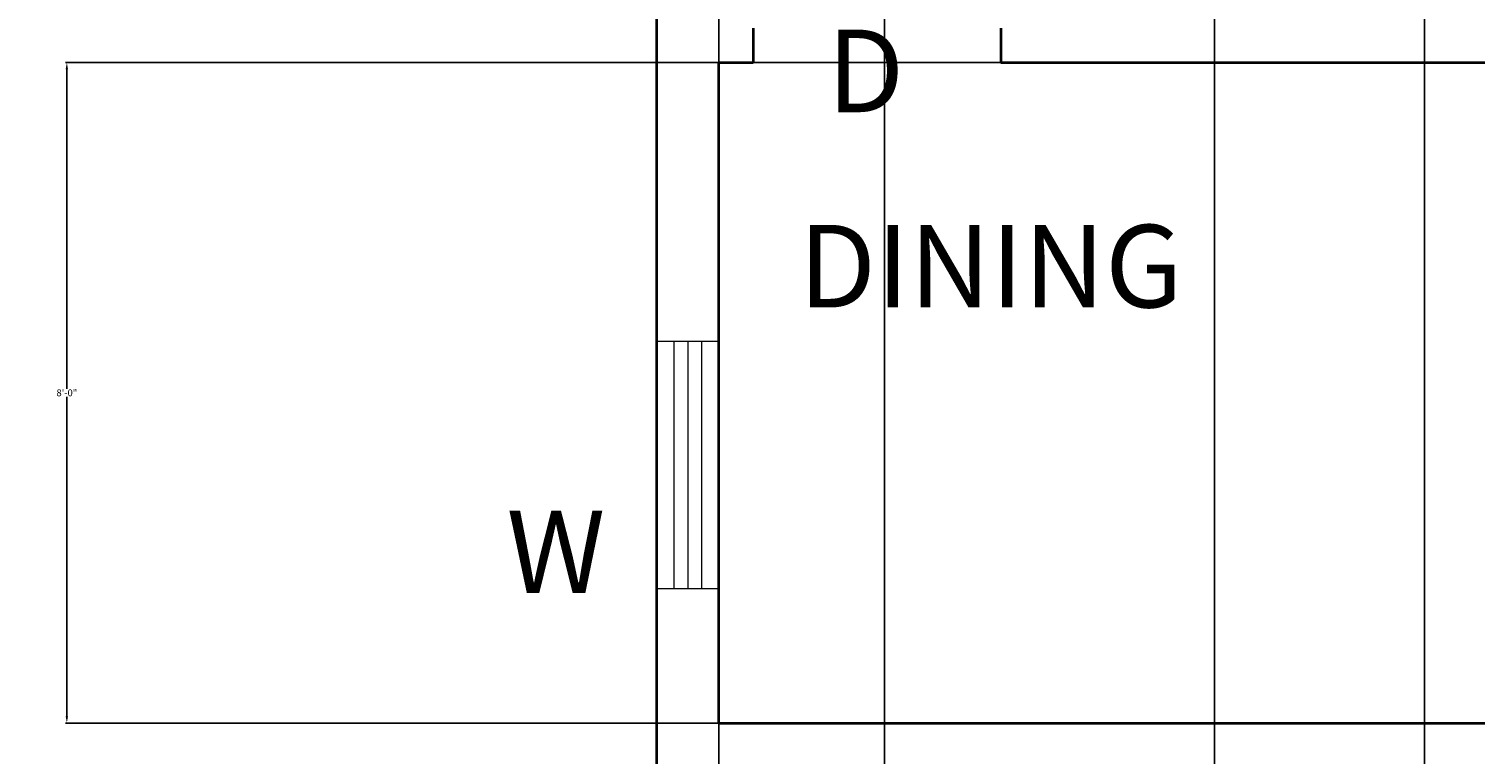
# Model space of a CAD drawing. Units: inches. Extents: x -304 to 580, y 363 to 1149.
# Tile 8 of 11: x -114 to 96, y 794 to 900. Entities that reach past the tile are written whole.
import ezdxf

# ---------------------------------------------------------------- set-up
doc = ezdxf.new("R2010")
doc.units = ezdxf.units.IN
doc.header["$MEASUREMENT"] = 0
for name, color, linetype, lineweight in [('A-ANNO-DIMS', 2, 'Continuous', 13), ('A-ANNO-IDEN', 7, 'Continuous', 18), ('A-AREA-IDEN', 7, 'Continuous', 25), ('A-GLAZ', 4, 'Continuous', 18), ('A-WALL', 40, 'Continuous', 35)]:
    doc.layers.add(name, color=color, linetype=linetype, lineweight=lineweight)
doc.styles.get("Standard").update_dxf_attribs({"font": 'arial.ttf'})
doc.dimstyles.get("Standard").update_dxf_attribs({"dimtxt": 1, "dimasz": 1, "dimexe": 0.18, "dimexo": 0.0625, "dimgap": 0.09, "dimtad": 0, "dimtih": 1, "dimtoh": 1, "dimdec": 0, "dimzin": 0, "dimdsep": 46, "dimlunit": 3, "dimtxsty": 'Standard', "dimcen": 0.09, "dimadec": 0, "dimazin": 0, "dimtfac": 1, "dimtdec": 0, "dimtofl": 0, "dimtmove": 0, "dimatfit": 3, "dimfxl": 1, "dimtolj": 1, "dimtzin": 0, "dimarcsym": 0})

# ---------------------------------------------------------------- blocks, each defined once
blk = doc.blocks.new('*D1')
at = {"layer": 'A-ANNO-DIMS', "color": 0, "lineweight": -2, "transparency": 16777216}
for p, q in [((-22.63, 1004.95), (-237.62, 1004.95)), ((-237.44, 1003.95), (-237.44, 721.93)), ((-237.44, 402.95), (-237.44, 684.96)), ((-22.63, 401.95), (-237.62, 401.95))]:
    blk.add_line(p, q, dxfattribs=at)
at = {"layer": 'A-ANNO-DIMS', "color": 0, "transparency": 16777216}
for points in [[(-237.61, 1003.95), (-237.28, 1003.95), (-237.44, 1004.95)], [(-237.61, 402.95), (-237.28, 402.95), (-237.44, 401.95)]]:
    blk.add_solid(points, dxfattribs=at)
at = {"layer": 'Defpoints', "color": 0, "transparency": 16777216}
for p in [(-22.57, 1004.95), (-237.44, 401.95), (-22.57, 401.95)]:
    blk.add_point(p, dxfattribs=at)
at = {"layer": 'A-ANNO-DIMS', "color": 0, "transparency": 16777216, "insert": (-237.44, 703.45), "char_height": 1, "attachment_point": 5}
blk.add_mtext('\\A1;{\\H36x;50\'-3"}', dxfattribs=at)
blk = doc.blocks.new('WIN-36IN')
for p, q in [((0, 6.5), (36, 6.5)), ((0, 4.5), (36, 4.5)), ((0, 2.5), (36, 2.5))]:
    blk.add_line(p, q)
blk.add_lwpolyline([(0, 0), (0, 9), (36, 9), (36, 0)], close=True)
blk = doc.blocks.new('*D33')
at = {"layer": 'A-ANNO-DIMS', "color": 0, "lineweight": -2, "transparency": 16777216}
for p, q in [((106.37, 894.95), (-108.5, 894.95)), ((-108.32, 893.95), (-108.32, 847.55)), ((-108.32, 799.95), (-108.32, 846.35)), ((106.37, 798.95), (-108.5, 798.95))]:
    blk.add_line(p, q, dxfattribs=at)
at = {"layer": 'A-ANNO-DIMS', "color": 0, "transparency": 16777216}
for points in [[(-108.49, 893.95), (-108.15, 893.95), (-108.32, 894.95)], [(-108.49, 799.95), (-108.15, 799.95), (-108.32, 798.95)]]:
    blk.add_solid(points, dxfattribs=at)
at = {"layer": 'Defpoints', "color": 0, "transparency": 16777216}
for p in [(-108.32, 894.95), (106.43, 894.95), (106.43, 798.95)]:
    blk.add_point(p, dxfattribs=at)
at = {"layer": 'A-ANNO-DIMS', "color": 0, "transparency": 16777216, "insert": (-108.32, 846.95), "char_height": 1, "attachment_point": 5}
blk.add_mtext('\\A1;8\'-0"', dxfattribs=at)
blk = doc.blocks.new('*D34')
at = {"layer": 'A-ANNO-DIMS', "color": 0, "lineweight": -2, "transparency": 16777216}
for p, q in [((10.51, 550.01), (10.51, 1042.88)), ((11.51, 1042.7), (33.07, 1042.7)), ((57.51, 1042.7), (35.95, 1042.7)), ((58.51, 550.01), (58.51, 1042.88))]:
    blk.add_line(p, q, dxfattribs=at)
at = {"layer": 'A-ANNO-DIMS', "color": 0, "transparency": 16777216}
for points in [[(11.51, 1042.86), (11.51, 1042.53), (10.51, 1042.7)], [(57.51, 1042.86), (57.51, 1042.53), (58.51, 1042.7)]]:
    blk.add_solid(points, dxfattribs=at)
at = {"layer": 'Defpoints', "color": 0, "transparency": 16777216}
for p in [(58.51, 1042.7), (10.51, 549.95), (58.51, 549.95)]:
    blk.add_point(p, dxfattribs=at)
at = {"layer": 'A-ANNO-DIMS', "color": 0, "transparency": 16777216, "insert": (34.51, 1042.7), "char_height": 1, "attachment_point": 5}
blk.add_mtext('\\A1;4\'-0"', dxfattribs=at)
blk = doc.blocks.new('*D35')
at = {"layer": 'A-ANNO-DIMS', "color": 0, "lineweight": -2, "transparency": 16777216}
for p, q in [((-13.57, 550.01), (-13.57, 1042.88)), ((-12.57, 1042.7), (-2.96, 1042.7)), ((9.51, 1042.7), (-0.1, 1042.7)), ((10.51, 550.01), (10.51, 1042.88))]:
    blk.add_line(p, q, dxfattribs=at)
at = {"layer": 'A-ANNO-DIMS', "color": 0, "transparency": 16777216}
for points in [[(-12.57, 1042.86), (-12.57, 1042.53), (-13.57, 1042.7)], [(9.51, 1042.86), (9.51, 1042.53), (10.51, 1042.7)]]:
    blk.add_solid(points, dxfattribs=at)
at = {"layer": 'Defpoints', "color": 0, "transparency": 16777216}
for p in [(10.51, 1042.7), (-13.57, 549.95), (10.51, 549.95)]:
    blk.add_point(p, dxfattribs=at)
at = {"layer": 'A-ANNO-DIMS', "color": 0, "transparency": 16777216, "insert": (-1.53, 1042.7), "char_height": 1, "attachment_point": 5}
blk.add_mtext('\\A1;2\'-0"', dxfattribs=at)
blk = doc.blocks.new('*D36')
at = {"layer": 'A-ANNO-DIMS', "color": 0, "lineweight": -2, "transparency": 16777216}
for p, q in [((-22.57, 516.57), (-22.57, 1042.88)), ((-21.57, 1042.7), (30.65, 1042.7)), ((88.04, 1042.7), (35.82, 1042.7)), ((89.04, 516.57), (89.04, 1042.88))]:
    blk.add_line(p, q, dxfattribs=at)
at = {"layer": 'A-ANNO-DIMS', "color": 0, "transparency": 16777216}
for points in [[(-21.57, 1042.86), (-21.57, 1042.53), (-22.57, 1042.7)], [(88.04, 1042.86), (88.04, 1042.53), (89.04, 1042.7)]]:
    blk.add_solid(points, dxfattribs=at)
at = {"layer": 'Defpoints', "color": 0, "transparency": 16777216}
for p in [(89.04, 1042.7), (-22.57, 516.51), (89.04, 516.51)]:
    blk.add_point(p, dxfattribs=at)
at = {"layer": 'A-ANNO-DIMS', "color": 0, "transparency": 16777216, "insert": (33.23, 1042.7), "char_height": 1, "attachment_point": 5}
blk.add_mtext('\\A1;9\'-3 1/2"', dxfattribs=at)

msp = doc.modelspace()

# ---------------------------------------------------------------- linework, layer by layer
at = {"layer": 'A-WALL'}
for p, q in [((-22.57, 516.51), (-22.57, 1004.95)), ((-8.57, 899.95), (-8.57, 894.95)), ((27.43, 899.95), (27.43, 894.95)), ((-13.57, 894.95), (-8.57, 894.95)), ((-13.57, 798.95), (-13.57, 894.95)), ((27.43, 894.95), (106.43, 894.95)), ((-13.57, 798.95), (106.43, 798.95))]:
    msp.add_line(p, q, dxfattribs=at)

# ---------------------------------------------------------------- block references
at = {"layer": 'A-GLAZ', "rotation": 270.0000000000001}
msp.add_blockref('WIN-36IN', (-22.57, 854.48), dxfattribs=at)

# ---------------------------------------------------------------- texts
at = {"layer": 'A-ANNO-IDEN', "char_height": 12, "attachment_point": 1}
for s, width, insert in [('D', 12.3109, (2.14, 899.73)), ('W', 41.6501, (-44.42, 829.84))]:
    msp.add_mtext_dynamic_manual_height_columns(s, width=width, gutter_width=1, heights=[0], dxfattribs=dict(at, insert=insert))
at = {"layer": 'A-AREA-IDEN', "insert": (-1.95, 871.36), "char_height": 12, "attachment_point": 1}
msp.add_mtext_dynamic_manual_height_columns('DINING', width=52.0965, gutter_width=1, heights=[0], dxfattribs=at)

# ---------------------------------------------------------------- dimensions: what is measured, and where the dimension line sits
at = {"layer": 'A-ANNO-DIMS'}
for base, p1, p2, picture, middle in [((89.04, 1042.7), (-22.57, 516.51), (89.04, 516.51), '*D36', (33.23, 1042.7)), ((10.51, 1042.7), (-13.57, 549.95), (10.51, 549.95), '*D35', (-1.53, 1042.7)), ((58.51, 1042.7), (10.51, 549.95), (58.51, 549.95), '*D34', (34.51, 1042.7))]:
    dim = msp.add_linear_dim(base=base, p1=p1, p2=p2, dimstyle='Standard', override={"dimdec": 1, "dimlfac": 1, "dimrnd": 0, "dimzin": 1, "dimdsep": 46, "dimlunit": 4, "dimfrac": 2}, dxfattribs=at)
    dim.commit()
    dim.dimension.update_dxf_attribs({"geometry": picture, "text_midpoint": middle})
dim = msp.add_linear_dim(base=(-237.44, 401.95), p1=(-22.57, 1004.95), p2=(-22.57, 401.95), angle=90, text='{\\H36x;<>}', dimstyle='Standard', override={"dimclrd": 0, "dimclre": 0, "dimclrt": 0}, dxfattribs=at)
dim.commit()
dim.dimension.update_dxf_attribs({"geometry": '*D1', "text_midpoint": (-237.44, 703.45)})
dim = msp.add_linear_dim(base=(-108.32, 894.95), p1=(106.43, 798.95), p2=(106.43, 894.95), angle=90, dimstyle='Standard', override={"dimdec": 1, "dimlfac": 1, "dimrnd": 0, "dimzin": 1, "dimdsep": 46, "dimlunit": 4, "dimfrac": 2}, dxfattribs=at)
dim.commit()
dim.dimension.update_dxf_attribs({"geometry": '*D33', "text_midpoint": (-108.32, 846.95)})

doc.saveas('drawing.dxf')
